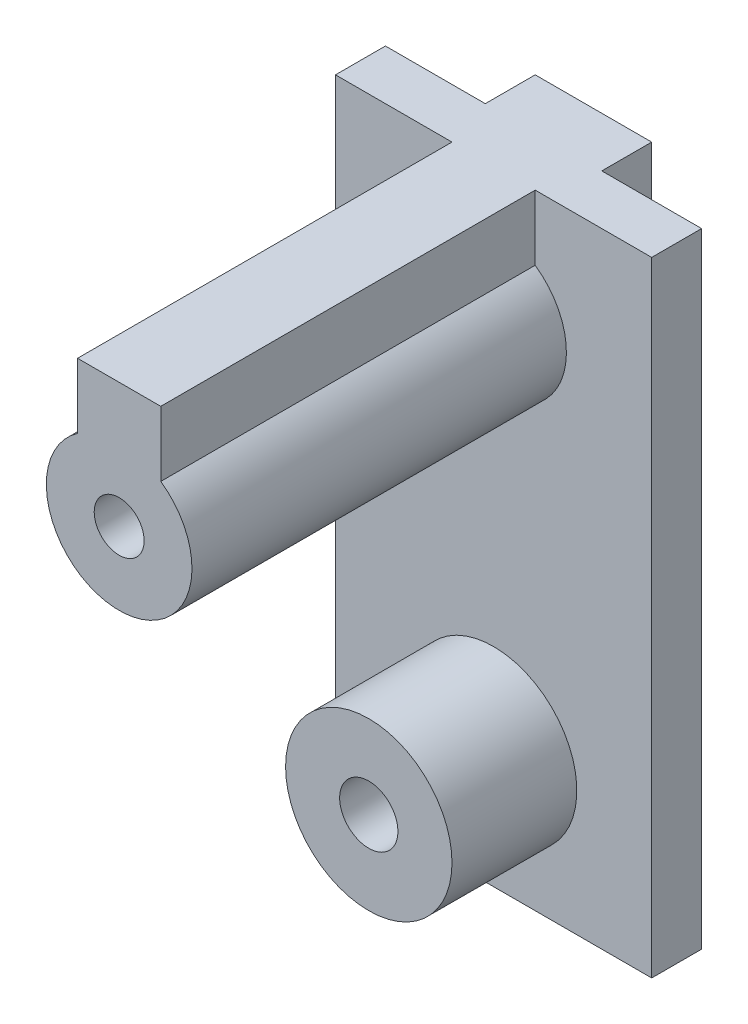
ISO-10303-21;
HEADER;
FILE_DESCRIPTION(('STEP AP214'),'2;1');
FILE_NAME('part.step','',(''),(''),'','','');
FILE_SCHEMA(('AUTOMOTIVE_DESIGN { 1 0 10303 214 1 1 1 1 }'));
ENDSEC;
DATA;
#1=APPLICATION_CONTEXT('core data for automotive mechanical design processes');
#2=APPLICATION_PROTOCOL_DEFINITION('international standard','automotive_design',2000,#1);
#3=PRODUCT_CONTEXT('',#1,'mechanical');
#4=PRODUCT('Part','Part','',(#3));
#5=PRODUCT_RELATED_PRODUCT_CATEGORY('part','',(#4));
#6=PRODUCT_DEFINITION_FORMATION('','',#4);
#7=PRODUCT_DEFINITION_CONTEXT('part definition',#1,'design');
#8=PRODUCT_DEFINITION('design','',#6,#7);
#9=PRODUCT_DEFINITION_SHAPE('','',#8);
#10=(LENGTH_UNIT() NAMED_UNIT(*) SI_UNIT(.MILLI.,.METRE.));
#11=(NAMED_UNIT(*) PLANE_ANGLE_UNIT() SI_UNIT($,.RADIAN.));
#12=(NAMED_UNIT(*) SI_UNIT($,.STERADIAN.) SOLID_ANGLE_UNIT());
#13=UNCERTAINTY_MEASURE_WITH_UNIT(LENGTH_MEASURE(1.E-05),#10,'distance_accuracy_value','');
#14=(GEOMETRIC_REPRESENTATION_CONTEXT(3) GLOBAL_UNCERTAINTY_ASSIGNED_CONTEXT((#13)) GLOBAL_UNIT_ASSIGNED_CONTEXT((#10,
#11,#12)) REPRESENTATION_CONTEXT('',''));
#15=CARTESIAN_POINT('',(0.,0.,0.));
#16=DIRECTION('',(0.,0.,1.));
#17=DIRECTION('',(1.,0.,0.));
#18=AXIS2_PLACEMENT_3D('',#15,#16,#17);
#19=CARTESIAN_POINT('',(0.,0.,0.));
#20=DIRECTION('',(0.,0.,-1.));
#21=DIRECTION('',(-1.,0.,0.));
#22=AXIS2_PLACEMENT_3D('',#19,#20,#21);
#23=PLANE('',#22);
#24=DIRECTION('',(-1.,0.,0.));
#25=VECTOR('',#24,1.);
#26=CARTESIAN_POINT('',(-38.,75.,0.));
#27=LINE('',#26,#25);
#28=CARTESIAN_POINT('',(-14.,75.,0.));
#29=VERTEX_POINT('',#28);
#30=CARTESIAN_POINT('',(-38.,75.,0.));
#31=VERTEX_POINT('',#30);
#32=EDGE_CURVE('E203',#29,#31,#27,.T.);
#33=ORIENTED_EDGE('',*,*,#32,.F.);
#34=DIRECTION('',(0.,-1.,0.));
#35=VECTOR('',#34,1.);
#36=CARTESIAN_POINT('',(-14.,75.,0.));
#37=LINE('',#36,#35);
#38=CARTESIAN_POINT('',(-14.,-75.,0.));
#39=VERTEX_POINT('',#38);
#40=EDGE_CURVE('E173',#29,#39,#37,.T.);
#41=ORIENTED_EDGE('',*,*,#40,.T.);
#42=DIRECTION('',(1.,0.,0.));
#43=VECTOR('',#42,1.);
#44=CARTESIAN_POINT('',(-38.,-75.,0.));
#45=LINE('',#44,#43);
#46=CARTESIAN_POINT('',(-38.,-75.,0.));
#47=VERTEX_POINT('',#46);
#48=EDGE_CURVE('E195',#47,#39,#45,.T.);
#49=ORIENTED_EDGE('',*,*,#48,.F.);
#50=DIRECTION('',(0.,-1.,0.));
#51=VECTOR('',#50,1.);
#52=CARTESIAN_POINT('',(-38.,-75.,0.));
#53=LINE('',#52,#51);
#54=EDGE_CURVE('E210',#31,#47,#53,.T.);
#55=ORIENTED_EDGE('',*,*,#54,.F.);
#56=EDGE_LOOP('',(#33,#41,#49,#55));
#57=FACE_BOUND('',#56,.T.);
#58=ADVANCED_FACE('F41',(#57),#23,.T.);
#59=CARTESIAN_POINT('',(38.,-75.,12.));
#60=DIRECTION('',(-1.,0.,0.));
#61=DIRECTION('',(0.,0.,1.));
#62=AXIS2_PLACEMENT_3D('',#59,#60,#61);
#63=PLANE('',#62);
#64=DIRECTION('',(0.,1.,0.));
#65=VECTOR('',#64,1.);
#66=CARTESIAN_POINT('',(38.,-75.,0.));
#67=LINE('',#66,#65);
#68=CARTESIAN_POINT('',(38.,-75.,0.));
#69=VERTEX_POINT('',#68);
#70=CARTESIAN_POINT('',(38.,75.,0.));
#71=VERTEX_POINT('',#70);
#72=EDGE_CURVE('E185',#69,#71,#67,.T.);
#73=ORIENTED_EDGE('',*,*,#72,.T.);
#74=DIRECTION('',(0.,0.,-1.));
#75=VECTOR('',#74,1.);
#76=CARTESIAN_POINT('',(38.,75.,12.));
#77=LINE('',#76,#75);
#78=CARTESIAN_POINT('',(38.,75.,12.));
#79=VERTEX_POINT('',#78);
#80=EDGE_CURVE('E219',#79,#71,#77,.T.);
#81=ORIENTED_EDGE('',*,*,#80,.F.);
#82=DIRECTION('',(0.,1.,0.));
#83=VECTOR('',#82,1.);
#84=CARTESIAN_POINT('',(38.,-75.,12.));
#85=LINE('',#84,#83);
#86=CARTESIAN_POINT('',(38.,-75.,12.));
#87=VERTEX_POINT('',#86);
#88=EDGE_CURVE('E189',#87,#79,#85,.T.);
#89=ORIENTED_EDGE('',*,*,#88,.F.);
#90=DIRECTION('',(0.,0.,-1.));
#91=VECTOR('',#90,1.);
#92=CARTESIAN_POINT('',(38.,-75.,12.));
#93=LINE('',#92,#91);
#94=EDGE_CURVE('E199',#87,#69,#93,.T.);
#95=ORIENTED_EDGE('',*,*,#94,.T.);
#96=EDGE_LOOP('',(#73,#81,#89,#95));
#97=FACE_BOUND('',#96,.T.);
#98=ADVANCED_FACE('F43',(#97),#63,.F.);
#99=CARTESIAN_POINT('',(-38.,75.,12.));
#100=DIRECTION('',(0.,-1.,0.));
#101=DIRECTION('',(0.,0.,-1.));
#102=AXIS2_PLACEMENT_3D('',#99,#100,#101);
#103=PLANE('',#102);
#104=CARTESIAN_POINT('',(14.,75.,0.));
#105=VERTEX_POINT('',#104);
#106=EDGE_CURVE('E204',#71,#105,#27,.T.);
#107=ORIENTED_EDGE('',*,*,#106,.T.);
#108=DIRECTION('',(0.,0.,1.));
#109=VECTOR('',#108,1.);
#110=CARTESIAN_POINT('',(14.,75.,-12.));
#111=LINE('',#110,#109);
#112=CARTESIAN_POINT('',(14.,75.,-12.));
#113=VERTEX_POINT('',#112);
#114=EDGE_CURVE('E171',#113,#105,#111,.T.);
#115=ORIENTED_EDGE('',*,*,#114,.F.);
#116=DIRECTION('',(1.,0.,0.));
#117=VECTOR('',#116,1.);
#118=CARTESIAN_POINT('',(-14.,75.,-12.));
#119=LINE('',#118,#117);
#120=CARTESIAN_POINT('',(-14.,75.,-12.));
#121=VERTEX_POINT('',#120);
#122=EDGE_CURVE('E170',#121,#113,#119,.T.);
#123=ORIENTED_EDGE('',*,*,#122,.F.);
#124=DIRECTION('',(0.,0.,-1.));
#125=VECTOR('',#124,1.);
#126=CARTESIAN_POINT('',(-14.,75.,0.));
#127=LINE('',#126,#125);
#128=EDGE_CURVE('E165',#29,#121,#127,.T.);
#129=ORIENTED_EDGE('',*,*,#128,.F.);
#130=ORIENTED_EDGE('',*,*,#32,.T.);
#131=DIRECTION('',(0.,0.,-1.));
#132=VECTOR('',#131,1.);
#133=CARTESIAN_POINT('',(-38.,75.,12.));
#134=LINE('',#133,#132);
#135=CARTESIAN_POINT('',(-38.,75.,12.));
#136=VERTEX_POINT('',#135);
#137=EDGE_CURVE('E220',#136,#31,#134,.T.);
#138=ORIENTED_EDGE('',*,*,#137,.F.);
#139=DIRECTION('',(-1.,0.,0.));
#140=VECTOR('',#139,1.);
#141=CARTESIAN_POINT('',(-38.,75.,12.));
#142=LINE('',#141,#140);
#143=CARTESIAN_POINT('',(-10.,75.,12.));
#144=VERTEX_POINT('',#143);
#145=EDGE_CURVE('E192',#144,#136,#142,.T.);
#146=ORIENTED_EDGE('',*,*,#145,.F.);
#147=DIRECTION('',(0.,0.,1.));
#148=VECTOR('',#147,1.);
#149=CARTESIAN_POINT('',(-10.,75.,12.));
#150=LINE('',#149,#148);
#151=CARTESIAN_POINT('',(-9.99999999999999,75.,102.));
#152=VERTEX_POINT('',#151);
#153=EDGE_CURVE('E286',#144,#152,#150,.T.);
#154=ORIENTED_EDGE('',*,*,#153,.T.);
#155=DIRECTION('',(1.,0.,0.));
#156=VECTOR('',#155,1.);
#157=CARTESIAN_POINT('',(-9.99999999999999,75.,102.));
#158=LINE('',#157,#156);
#159=CARTESIAN_POINT('',(9.99999999999999,75.,102.));
#160=VERTEX_POINT('',#159);
#161=EDGE_CURVE('E145',#152,#160,#158,.T.);
#162=ORIENTED_EDGE('',*,*,#161,.T.);
#163=DIRECTION('',(0.,0.,-1.));
#164=VECTOR('',#163,1.);
#165=CARTESIAN_POINT('',(10.,75.,12.));
#166=LINE('',#165,#164);
#167=CARTESIAN_POINT('',(10.,75.,12.));
#168=VERTEX_POINT('',#167);
#169=EDGE_CURVE('E296',#160,#168,#166,.T.);
#170=ORIENTED_EDGE('',*,*,#169,.T.);
#171=EDGE_CURVE('E194',#79,#168,#142,.T.);
#172=ORIENTED_EDGE('',*,*,#171,.F.);
#173=ORIENTED_EDGE('',*,*,#80,.T.);
#174=EDGE_LOOP('',(#107,#115,#123,#129,#130,#138,#146,#154,#162,#170,#172,#173));
#175=FACE_BOUND('',#174,.T.);
#176=ADVANCED_FACE('F261',(#175),#103,.F.);
#177=CARTESIAN_POINT('',(-38.,-75.,12.));
#178=DIRECTION('',(1.,0.,0.));
#179=DIRECTION('',(0.,0.,-1.));
#180=AXIS2_PLACEMENT_3D('',#177,#178,#179);
#181=PLANE('',#180);
#182=ORIENTED_EDGE('',*,*,#54,.T.);
#183=DIRECTION('',(0.,0.,-1.));
#184=VECTOR('',#183,1.);
#185=CARTESIAN_POINT('',(-38.,-75.,12.));
#186=LINE('',#185,#184);
#187=CARTESIAN_POINT('',(-38.,-75.,12.));
#188=VERTEX_POINT('',#187);
#189=EDGE_CURVE('E211',#188,#47,#186,.T.);
#190=ORIENTED_EDGE('',*,*,#189,.F.);
#191=DIRECTION('',(0.,-1.,0.));
#192=VECTOR('',#191,1.);
#193=CARTESIAN_POINT('',(-38.,-75.,12.));
#194=LINE('',#193,#192);
#195=EDGE_CURVE('E196',#136,#188,#194,.T.);
#196=ORIENTED_EDGE('',*,*,#195,.F.);
#197=ORIENTED_EDGE('',*,*,#137,.T.);
#198=EDGE_LOOP('',(#182,#190,#196,#197));
#199=FACE_BOUND('',#198,.T.);
#200=ADVANCED_FACE('F242',(#199),#181,.F.);
#201=CARTESIAN_POINT('',(-38.,-75.,12.));
#202=DIRECTION('',(0.,1.,0.));
#203=DIRECTION('',(0.,0.,1.));
#204=AXIS2_PLACEMENT_3D('',#201,#202,#203);
#205=PLANE('',#204);
#206=ORIENTED_EDGE('',*,*,#48,.T.);
#207=DIRECTION('',(0.,0.,-1.));
#208=VECTOR('',#207,1.);
#209=CARTESIAN_POINT('',(-14.,-75.,0.));
#210=LINE('',#209,#208);
#211=CARTESIAN_POINT('',(-14.,-75.,-12.));
#212=VERTEX_POINT('',#211);
#213=EDGE_CURVE('E61',#39,#212,#210,.T.);
#214=ORIENTED_EDGE('',*,*,#213,.T.);
#215=DIRECTION('',(1.,0.,0.));
#216=VECTOR('',#215,1.);
#217=CARTESIAN_POINT('',(-14.,-75.,-12.));
#218=LINE('',#217,#216);
#219=CARTESIAN_POINT('',(14.,-75.,-12.));
#220=VERTEX_POINT('',#219);
#221=EDGE_CURVE('E174',#212,#220,#218,.T.);
#222=ORIENTED_EDGE('',*,*,#221,.T.);
#223=DIRECTION('',(0.,0.,1.));
#224=VECTOR('',#223,1.);
#225=CARTESIAN_POINT('',(14.,-75.,-12.));
#226=LINE('',#225,#224);
#227=CARTESIAN_POINT('',(14.,-75.,0.));
#228=VERTEX_POINT('',#227);
#229=EDGE_CURVE('E166',#220,#228,#226,.T.);
#230=ORIENTED_EDGE('',*,*,#229,.T.);
#231=EDGE_CURVE('E209',#228,#69,#45,.T.);
#232=ORIENTED_EDGE('',*,*,#231,.T.);
#233=ORIENTED_EDGE('',*,*,#94,.F.);
#234=DIRECTION('',(1.,0.,0.));
#235=VECTOR('',#234,1.);
#236=CARTESIAN_POINT('',(-38.,-75.,12.));
#237=LINE('',#236,#235);
#238=EDGE_CURVE('E198',#188,#87,#237,.T.);
#239=ORIENTED_EDGE('',*,*,#238,.F.);
#240=ORIENTED_EDGE('',*,*,#189,.T.);
#241=EDGE_LOOP('',(#206,#214,#222,#230,#232,#233,#239,#240));
#242=FACE_BOUND('',#241,.T.);
#243=ADVANCED_FACE('F229',(#242),#205,.F.);
#244=CARTESIAN_POINT('',(0.,0.,12.));
#245=DIRECTION('',(0.,0.,-1.));
#246=DIRECTION('',(-1.,0.,0.));
#247=AXIS2_PLACEMENT_3D('',#244,#245,#246);
#248=PLANE('',#247);
#249=ORIENTED_EDGE('',*,*,#171,.T.);
#250=DIRECTION('',(0.,1.,0.));
#251=VECTOR('',#250,1.);
#252=CARTESIAN_POINT('',(10.,-75.001,12.));
#253=LINE('',#252,#251);
#254=CARTESIAN_POINT('',(9.99999999999999,59.3614066163451,12.));
#255=VERTEX_POINT('',#254);
#256=EDGE_CURVE('E292',#255,#168,#253,.T.);
#257=ORIENTED_EDGE('',*,*,#256,.F.);
#258=CARTESIAN_POINT('',(0.,45.,12.));
#259=DIRECTION('',(0.,0.,-1.));
#260=DIRECTION('',(-1.,0.,0.));
#261=AXIS2_PLACEMENT_3D('',#258,#259,#260);
#262=CIRCLE('',#261,17.5);
#263=CARTESIAN_POINT('',(-9.99999999999999,59.3614066163451,12.));
#264=VERTEX_POINT('',#263);
#265=EDGE_CURVE('E11',#264,#255,#262,.F.);
#266=ORIENTED_EDGE('',*,*,#265,.F.);
#267=DIRECTION('',(0.,1.,0.));
#268=VECTOR('',#267,1.);
#269=CARTESIAN_POINT('',(-10.,-75.001,12.));
#270=LINE('',#269,#268);
#271=EDGE_CURVE('E57',#264,#144,#270,.T.);
#272=ORIENTED_EDGE('',*,*,#271,.T.);
#273=ORIENTED_EDGE('',*,*,#145,.T.);
#274=ORIENTED_EDGE('',*,*,#195,.T.);
#275=ORIENTED_EDGE('',*,*,#238,.T.);
#276=ORIENTED_EDGE('',*,*,#88,.T.);
#277=EDGE_LOOP('',(#249,#257,#266,#272,#273,#274,#275,#276));
#278=FACE_BOUND('',#277,.T.);
#279=CARTESIAN_POINT('',(0.,-45.,12.));
#280=DIRECTION('',(0.,0.,-1.));
#281=DIRECTION('',(-1.,0.,0.));
#282=AXIS2_PLACEMENT_3D('',#279,#280,#281);
#283=CIRCLE('',#282,20.);
#284=CARTESIAN_POINT('',(-20.,-45.,12.));
#285=VERTEX_POINT('',#284);
#286=EDGE_CURVE('E47',#285,#285,#283,.F.);
#287=ORIENTED_EDGE('',*,*,#286,.F.);
#288=EDGE_LOOP('',(#287));
#289=FACE_BOUND('',#288,.T.);
#290=ADVANCED_FACE('F227',(#278,#289),#248,.F.);
#291=DIRECTION('',(0.,-1.,0.));
#292=VECTOR('',#291,1.);
#293=CARTESIAN_POINT('',(14.,75.,0.));
#294=LINE('',#293,#292);
#295=EDGE_CURVE('E179',#105,#228,#294,.T.);
#296=ORIENTED_EDGE('',*,*,#295,.F.);
#297=ORIENTED_EDGE('',*,*,#106,.F.);
#298=ORIENTED_EDGE('',*,*,#72,.F.);
#299=ORIENTED_EDGE('',*,*,#231,.F.);
#300=EDGE_LOOP('',(#296,#297,#298,#299));
#301=FACE_BOUND('',#300,.T.);
#302=ADVANCED_FACE('F230',(#301),#23,.T.);
#303=CARTESIAN_POINT('',(14.,75.,-12.));
#304=DIRECTION('',(1.,0.,0.));
#305=DIRECTION('',(0.,0.,-1.));
#306=AXIS2_PLACEMENT_3D('',#303,#304,#305);
#307=PLANE('',#306);
#308=ORIENTED_EDGE('',*,*,#229,.F.);
#309=DIRECTION('',(0.,-1.,0.));
#310=VECTOR('',#309,1.);
#311=CARTESIAN_POINT('',(14.,75.,-12.));
#312=LINE('',#311,#310);
#313=EDGE_CURVE('E182',#113,#220,#312,.T.);
#314=ORIENTED_EDGE('',*,*,#313,.F.);
#315=ORIENTED_EDGE('',*,*,#114,.T.);
#316=ORIENTED_EDGE('',*,*,#295,.T.);
#317=EDGE_LOOP('',(#308,#314,#315,#316));
#318=FACE_BOUND('',#317,.T.);
#319=ADVANCED_FACE('F239',(#318),#307,.T.);
#320=CARTESIAN_POINT('',(-14.,75.,-12.));
#321=DIRECTION('',(0.,0.,-1.));
#322=DIRECTION('',(-1.,0.,0.));
#323=AXIS2_PLACEMENT_3D('',#320,#321,#322);
#324=PLANE('',#323);
#325=ORIENTED_EDGE('',*,*,#221,.F.);
#326=DIRECTION('',(0.,-1.,0.));
#327=VECTOR('',#326,1.);
#328=CARTESIAN_POINT('',(-14.,75.,-12.));
#329=LINE('',#328,#327);
#330=EDGE_CURVE('E184',#121,#212,#329,.T.);
#331=ORIENTED_EDGE('',*,*,#330,.F.);
#332=ORIENTED_EDGE('',*,*,#122,.T.);
#333=ORIENTED_EDGE('',*,*,#313,.T.);
#334=EDGE_LOOP('',(#325,#331,#332,#333));
#335=FACE_BOUND('',#334,.T.);
#336=ADVANCED_FACE('F278',(#335),#324,.T.);
#337=CARTESIAN_POINT('',(-14.,75.,0.));
#338=DIRECTION('',(-1.,0.,0.));
#339=DIRECTION('',(0.,0.,1.));
#340=AXIS2_PLACEMENT_3D('',#337,#338,#339);
#341=PLANE('',#340);
#342=ORIENTED_EDGE('',*,*,#213,.F.);
#343=ORIENTED_EDGE('',*,*,#40,.F.);
#344=ORIENTED_EDGE('',*,*,#128,.T.);
#345=ORIENTED_EDGE('',*,*,#330,.T.);
#346=EDGE_LOOP('',(#342,#343,#344,#345));
#347=FACE_BOUND('',#346,.T.);
#348=ADVANCED_FACE('F285',(#347),#341,.T.);
#349=CARTESIAN_POINT('',(0.,-45.,42.));
#350=DIRECTION('',(0.,0.,-1.));
#351=DIRECTION('',(-1.,0.,0.));
#352=AXIS2_PLACEMENT_3D('',#349,#350,#351);
#353=CYLINDRICAL_SURFACE('',#352,7.);
#354=CARTESIAN_POINT('',(0.,-45.,42.));
#355=DIRECTION('',(0.,0.,1.));
#356=DIRECTION('',(1.,0.,0.));
#357=AXIS2_PLACEMENT_3D('',#354,#355,#356);
#358=CIRCLE('',#357,7.);
#359=CARTESIAN_POINT('',(7.,-45.,42.));
#360=VERTEX_POINT('',#359);
#361=EDGE_CURVE('E153',#360,#360,#358,.T.);
#362=ORIENTED_EDGE('',*,*,#361,.T.);
#363=EDGE_LOOP('',(#362));
#364=FACE_BOUND('',#363,.T.);
#365=CARTESIAN_POINT('',(0.,-45.,12.));
#366=DIRECTION('',(0.,0.,1.));
#367=DIRECTION('',(1.,0.,0.));
#368=AXIS2_PLACEMENT_3D('',#365,#366,#367);
#369=CIRCLE('',#368,7.);
#370=CARTESIAN_POINT('',(7.,-45.,12.));
#371=VERTEX_POINT('',#370);
#372=EDGE_CURVE('E146',#371,#371,#369,.T.);
#373=ORIENTED_EDGE('',*,*,#372,.F.);
#374=EDGE_LOOP('',(#373));
#375=FACE_BOUND('',#374,.T.);
#376=ADVANCED_FACE('F321',(#364,#375),#353,.F.);
#377=CARTESIAN_POINT('',(0.,-45.,42.));
#378=DIRECTION('',(0.,0.,-1.));
#379=DIRECTION('',(-1.,0.,0.));
#380=AXIS2_PLACEMENT_3D('',#377,#378,#379);
#381=CYLINDRICAL_SURFACE('',#380,20.);
#382=CARTESIAN_POINT('',(0.,-45.,42.));
#383=DIRECTION('',(0.,0.,1.));
#384=DIRECTION('',(1.,0.,0.));
#385=AXIS2_PLACEMENT_3D('',#382,#383,#384);
#386=CIRCLE('',#385,20.);
#387=CARTESIAN_POINT('',(20.,-45.,42.));
#388=VERTEX_POINT('',#387);
#389=EDGE_CURVE('E163',#388,#388,#386,.T.);
#390=ORIENTED_EDGE('',*,*,#389,.F.);
#391=EDGE_LOOP('',(#390));
#392=FACE_BOUND('',#391,.T.);
#393=ORIENTED_EDGE('',*,*,#286,.T.);
#394=EDGE_LOOP('',(#393));
#395=FACE_BOUND('',#394,.T.);
#396=ADVANCED_FACE('F221',(#392,#395),#381,.T.);
#397=CARTESIAN_POINT('',(0.,0.,42.));
#398=DIRECTION('',(0.,0.,1.));
#399=DIRECTION('',(1.,0.,0.));
#400=AXIS2_PLACEMENT_3D('',#397,#398,#399);
#401=PLANE('',#400);
#402=ORIENTED_EDGE('',*,*,#361,.F.);
#403=EDGE_LOOP('',(#402));
#404=FACE_BOUND('',#403,.T.);
#405=ORIENTED_EDGE('',*,*,#389,.T.);
#406=EDGE_LOOP('',(#405));
#407=FACE_BOUND('',#406,.T.);
#408=ADVANCED_FACE('F254',(#404,#407),#401,.T.);
#409=ORIENTED_EDGE('',*,*,#372,.T.);
#410=EDGE_LOOP('',(#409));
#411=FACE_BOUND('',#410,.T.);
#412=ADVANCED_FACE('F234',(#411),#248,.F.);
#413=CARTESIAN_POINT('',(0.,45.,102.));
#414=DIRECTION('',(0.,0.,1.));
#415=DIRECTION('',(1.,0.,0.));
#416=AXIS2_PLACEMENT_3D('',#413,#414,#415);
#417=PLANE('',#416);
#418=CARTESIAN_POINT('',(0.,45.,102.));
#419=DIRECTION('',(0.,0.,1.));
#420=DIRECTION('',(1.,0.,0.));
#421=AXIS2_PLACEMENT_3D('',#418,#419,#420);
#422=CIRCLE('',#421,17.5);
#423=CARTESIAN_POINT('',(-9.99999999999999,59.3614066163451,102.));
#424=VERTEX_POINT('',#423);
#425=CARTESIAN_POINT('',(9.99999999999999,59.3614066163451,102.));
#426=VERTEX_POINT('',#425);
#427=EDGE_CURVE('E136',#424,#426,#422,.T.);
#428=ORIENTED_EDGE('',*,*,#427,.T.);
#429=DIRECTION('',(0.,1.,0.));
#430=VECTOR('',#429,1.);
#431=CARTESIAN_POINT('',(9.99999999999999,-75.001,102.));
#432=LINE('',#431,#430);
#433=EDGE_CURVE('E300',#426,#160,#432,.T.);
#434=ORIENTED_EDGE('',*,*,#433,.T.);
#435=ORIENTED_EDGE('',*,*,#161,.F.);
#436=DIRECTION('',(0.,1.,0.));
#437=VECTOR('',#436,1.);
#438=CARTESIAN_POINT('',(-9.99999999999999,-75.001,102.));
#439=LINE('',#438,#437);
#440=EDGE_CURVE('E128',#424,#152,#439,.T.);
#441=ORIENTED_EDGE('',*,*,#440,.F.);
#442=EDGE_LOOP('',(#428,#434,#435,#441));
#443=FACE_BOUND('',#442,.T.);
#444=CARTESIAN_POINT('',(0.,45.,102.));
#445=DIRECTION('',(0.,0.,1.));
#446=DIRECTION('',(1.,0.,0.));
#447=AXIS2_PLACEMENT_3D('',#444,#445,#446);
#448=CIRCLE('',#447,6.);
#449=CARTESIAN_POINT('',(-6.,45.,102.));
#450=VERTEX_POINT('',#449);
#451=EDGE_CURVE('E148',#450,#450,#448,.T.);
#452=ORIENTED_EDGE('',*,*,#451,.F.);
#453=EDGE_LOOP('',(#452));
#454=FACE_BOUND('',#453,.T.);
#455=ADVANCED_FACE('F138',(#443,#454),#417,.T.);
#456=CARTESIAN_POINT('',(0.,45.,102.));
#457=DIRECTION('',(0.,0.,-1.));
#458=DIRECTION('',(-1.,0.,0.));
#459=AXIS2_PLACEMENT_3D('',#456,#457,#458);
#460=CYLINDRICAL_SURFACE('',#459,17.5);
#461=ORIENTED_EDGE('',*,*,#265,.T.);
#462=DIRECTION('',(0.,0.,-1.));
#463=VECTOR('',#462,1.);
#464=CARTESIAN_POINT('',(9.99999999999999,59.3614066163451,102.));
#465=LINE('',#464,#463);
#466=EDGE_CURVE('E149',#426,#255,#465,.T.);
#467=ORIENTED_EDGE('',*,*,#466,.F.);
#468=ORIENTED_EDGE('',*,*,#427,.F.);
#469=DIRECTION('',(0.,0.,-1.));
#470=VECTOR('',#469,1.);
#471=CARTESIAN_POINT('',(-9.99999999999999,59.3614066163451,102.));
#472=LINE('',#471,#470);
#473=EDGE_CURVE('E130',#264,#424,#472,.F.);
#474=ORIENTED_EDGE('',*,*,#473,.F.);
#475=EDGE_LOOP('',(#461,#467,#468,#474));
#476=FACE_BOUND('',#475,.T.);
#477=ADVANCED_FACE('F150',(#476),#460,.T.);
#478=CARTESIAN_POINT('',(0.,45.,102.));
#479=DIRECTION('',(0.,0.,-1.));
#480=DIRECTION('',(-1.,0.,0.));
#481=AXIS2_PLACEMENT_3D('',#478,#479,#480);
#482=CYLINDRICAL_SURFACE('',#481,6.);
#483=CARTESIAN_POINT('',(0.,45.,12.));
#484=DIRECTION('',(0.,0.,1.));
#485=DIRECTION('',(1.,0.,0.));
#486=AXIS2_PLACEMENT_3D('',#483,#484,#485);
#487=CIRCLE('',#486,6.);
#488=CARTESIAN_POINT('',(-6.,45.,12.));
#489=VERTEX_POINT('',#488);
#490=EDGE_CURVE('E144',#489,#489,#487,.T.);
#491=CARTESIAN_POINT('',(-6.,45.,102.));
#492=CARTESIAN_POINT('',(-6.,45.,101.0625));
#493=CARTESIAN_POINT('',(-6.,45.,100.125));
#494=CARTESIAN_POINT('',(-6.,45.,98.25));
#495=CARTESIAN_POINT('',(-6.,45.,97.3125));
#496=CARTESIAN_POINT('',(-6.,45.,95.4375));
#497=CARTESIAN_POINT('',(-6.,45.,94.5));
#498=CARTESIAN_POINT('',(-6.,45.,92.625));
#499=CARTESIAN_POINT('',(-6.,45.,91.6875));
#500=CARTESIAN_POINT('',(-6.,45.,89.8125));
#501=CARTESIAN_POINT('',(-6.,45.,88.875));
#502=CARTESIAN_POINT('',(-6.,45.,87.));
#503=CARTESIAN_POINT('',(-6.,45.,86.0625));
#504=CARTESIAN_POINT('',(-6.,45.,84.1875));
#505=CARTESIAN_POINT('',(-6.,45.,83.25));
#506=CARTESIAN_POINT('',(-6.,45.,81.375));
#507=CARTESIAN_POINT('',(-6.,45.,80.4375));
#508=CARTESIAN_POINT('',(-6.,45.,78.5625));
#509=CARTESIAN_POINT('',(-6.,45.,77.625));
#510=CARTESIAN_POINT('',(-6.,45.,75.75));
#511=CARTESIAN_POINT('',(-6.,45.,74.8125));
#512=CARTESIAN_POINT('',(-6.,45.,72.9375));
#513=CARTESIAN_POINT('',(-6.,45.,72.));
#514=CARTESIAN_POINT('',(-6.,45.,70.125));
#515=CARTESIAN_POINT('',(-6.,45.,69.1875));
#516=CARTESIAN_POINT('',(-6.,45.,67.3125));
#517=CARTESIAN_POINT('',(-6.,45.,66.375));
#518=CARTESIAN_POINT('',(-6.,45.,64.5));
#519=CARTESIAN_POINT('',(-6.,45.,63.5625));
#520=CARTESIAN_POINT('',(-6.,45.,61.6875));
#521=CARTESIAN_POINT('',(-6.,45.,60.75));
#522=CARTESIAN_POINT('',(-6.,45.,58.875));
#523=CARTESIAN_POINT('',(-6.,45.,57.9375));
#524=CARTESIAN_POINT('',(-6.,45.,56.0625));
#525=CARTESIAN_POINT('',(-6.,45.,55.125));
#526=CARTESIAN_POINT('',(-6.,45.,53.25));
#527=CARTESIAN_POINT('',(-6.,45.,52.3125));
#528=CARTESIAN_POINT('',(-6.,45.,50.4375));
#529=CARTESIAN_POINT('',(-6.,45.,49.5));
#530=CARTESIAN_POINT('',(-6.,45.,47.625));
#531=CARTESIAN_POINT('',(-6.,45.,46.6875));
#532=CARTESIAN_POINT('',(-6.,45.,44.8125));
#533=CARTESIAN_POINT('',(-6.,45.,43.875));
#534=CARTESIAN_POINT('',(-6.,45.,42.));
#535=CARTESIAN_POINT('',(-6.,45.,41.0625));
#536=CARTESIAN_POINT('',(-6.,45.,39.1875));
#537=CARTESIAN_POINT('',(-6.,45.,38.25));
#538=CARTESIAN_POINT('',(-6.,45.,36.375));
#539=CARTESIAN_POINT('',(-6.,45.,35.4375));
#540=CARTESIAN_POINT('',(-6.,45.,33.5625));
#541=CARTESIAN_POINT('',(-6.,45.,32.625));
#542=CARTESIAN_POINT('',(-6.,45.,30.75));
#543=CARTESIAN_POINT('',(-6.,45.,29.8125));
#544=CARTESIAN_POINT('',(-6.,45.,27.9375));
#545=CARTESIAN_POINT('',(-6.,45.,27.));
#546=CARTESIAN_POINT('',(-6.,45.,25.125));
#547=CARTESIAN_POINT('',(-6.,45.,24.1875));
#548=CARTESIAN_POINT('',(-6.,45.,22.3125));
#549=CARTESIAN_POINT('',(-6.,45.,21.375));
#550=CARTESIAN_POINT('',(-6.,45.,19.5));
#551=CARTESIAN_POINT('',(-6.,45.,18.5625));
#552=CARTESIAN_POINT('',(-6.,45.,16.6875));
#553=CARTESIAN_POINT('',(-6.,45.,15.75));
#554=CARTESIAN_POINT('',(-6.,45.,13.875));
#555=CARTESIAN_POINT('',(-6.,45.,12.9375));
#556=CARTESIAN_POINT('',(-6.,45.,12.));
#557=B_SPLINE_CURVE_WITH_KNOTS('',3,(#491,#492,#493,#494,#495,#496,#497,#498,#499,#500,#501,
#502,#503,#504,#505,#506,#507,#508,#509,#510,#511,#512,#513,#514,#515,#516,#517,#518,#519,#520,
#521,#522,#523,#524,#525,#526,#527,#528,#529,#530,#531,#532,#533,#534,#535,#536,#537,#538,#539,
#540,#541,#542,#543,#544,#545,#546,#547,#548,#549,#550,#551,#552,#553,#554,#555,#556),
.UNSPECIFIED.,.F.,.F.,(4,2,2,2,2,2,2,2,2,2,2,2,2,2,2,2,2,2,2,2,2,2,2,2,2,2,2,2,2,2,2,2,4),(0.,
2.81250000000001,5.62500000000001,8.4375,11.25,14.0625,16.875,19.6875,22.5,25.3125,28.125,
30.9375,33.75,36.5625,39.375,42.1875,45.,47.8125,50.625,53.4375,56.25,59.0625,61.875,64.6875,
67.5,70.3125,73.125,75.9375,78.75,81.5625,84.375,87.1875,90.),.UNSPECIFIED.);
#558=EDGE_CURVE('BSEAM249',#450,#489,#557,.T.);
#559=ORIENTED_EDGE('',*,*,#451,.T.);
#560=ORIENTED_EDGE('',*,*,#490,.F.);
#561=ORIENTED_EDGE('',*,*,#558,.T.);
#562=ORIENTED_EDGE('',*,*,#558,.F.);
#563=EDGE_LOOP('',(#559,#561,#560,#562));
#564=FACE_BOUND('',#563,.T.);
#565=ADVANCED_FACE('F249',(#564),#482,.F.);
#566=ORIENTED_EDGE('',*,*,#490,.T.);
#567=EDGE_LOOP('',(#566));
#568=FACE_BOUND('',#567,.T.);
#569=ADVANCED_FACE('F231',(#568),#248,.F.);
#570=CARTESIAN_POINT('',(10.,-75.001,12.));
#571=DIRECTION('',(1.,0.,0.));
#572=DIRECTION('',(0.,0.,-1.));
#573=AXIS2_PLACEMENT_3D('',#570,#571,#572);
#574=PLANE('',#573);
#575=ORIENTED_EDGE('',*,*,#433,.F.);
#576=ORIENTED_EDGE('',*,*,#466,.T.);
#577=ORIENTED_EDGE('',*,*,#256,.T.);
#578=ORIENTED_EDGE('',*,*,#169,.F.);
#579=EDGE_LOOP('',(#575,#576,#577,#578));
#580=FACE_BOUND('',#579,.T.);
#581=ADVANCED_FACE('F248',(#580),#574,.T.);
#582=CARTESIAN_POINT('',(-10.,-75.001,12.));
#583=DIRECTION('',(-1.,0.,0.));
#584=DIRECTION('',(0.,0.,1.));
#585=AXIS2_PLACEMENT_3D('',#582,#583,#584);
#586=PLANE('',#585);
#587=ORIENTED_EDGE('',*,*,#271,.F.);
#588=ORIENTED_EDGE('',*,*,#473,.T.);
#589=ORIENTED_EDGE('',*,*,#440,.T.);
#590=ORIENTED_EDGE('',*,*,#153,.F.);
#591=EDGE_LOOP('',(#587,#588,#589,#590));
#592=FACE_BOUND('',#591,.T.);
#593=ADVANCED_FACE('F126',(#592),#586,.T.);
#594=CLOSED_SHELL('',(#58,#98,#176,#200,#243,#290,#302,#319,#336,#348,#376,#396,#408,#412,#455,
#477,#565,#569,#581,#593));
#595=MANIFOLD_SOLID_BREP('B2',#594);
#596=ADVANCED_BREP_SHAPE_REPRESENTATION('',(#18,#595),#14);
#597=SHAPE_DEFINITION_REPRESENTATION(#9,#596);
ENDSEC;
END-ISO-10303-21;
